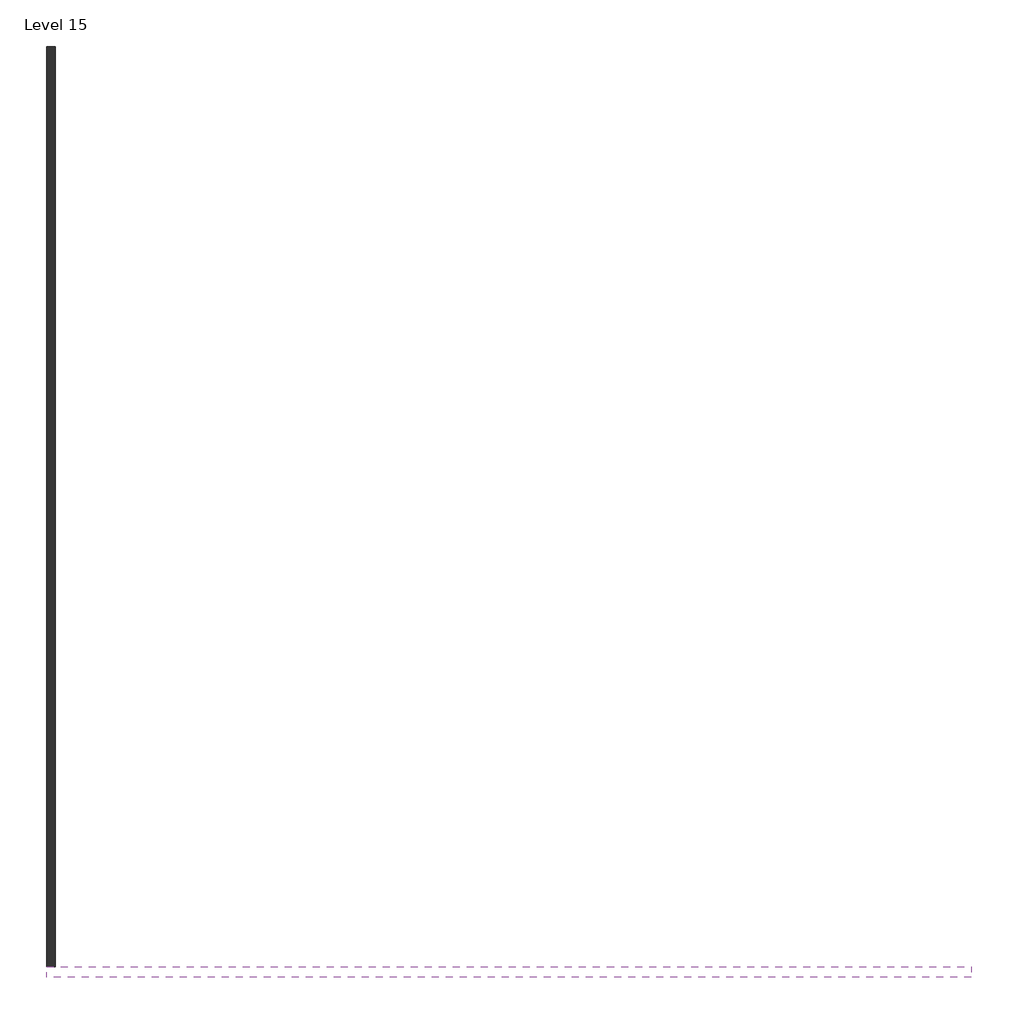
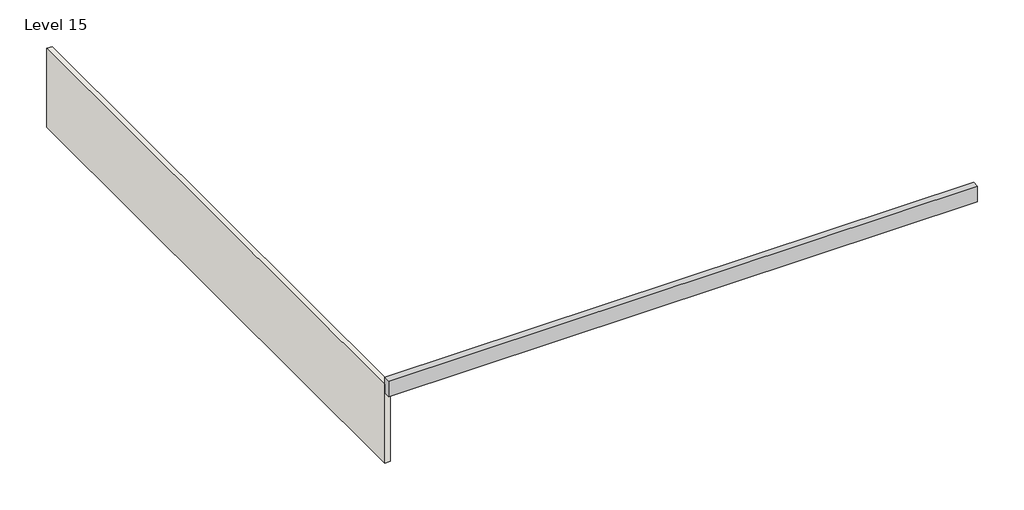
# One storey: 1 proxy, 1 wall.
"""IFC4 building model written with IfcOpenShell, lengths in millimetres."""

from ifc_helpers import new_model, si_unit, origin, place, context, project, spatial, faceted_brep, transform, mapped, element, save
from components import generic_models_10_generic_models_10_516a4994

model = new_model("IFC4")

# Units and contexts
model_context = context("Model", 3, world=origin())
ifc_project = project(units=[si_unit("LENGTHUNIT", "METRE", prefix="MILLI")], contexts=[model_context])

# Site, building, storey
site = spatial("IfcSite", under=ifc_project)
building = spatial("IfcBuilding", under=site)
storey = spatial("IfcBuildingStorey", under=building, Name="Level 15", Elevation=22936.2)

# Proxy
placement = place(None, origin())
generic_models_10_generic_models_10_shape = generic_models_10_generic_models_10_516a4994(model_context)
element("IfcBuildingElementProxy", 1, Name="Generic Models 10 : Generic Models 10", ObjectType="Generic Models 10 : Generic Models 10", at=placement, inside=storey, context=model_context, shape_type="MappedRepresentation", body=[
    mapped(generic_models_10_generic_models_10_shape, transform((0.0, 0.0, 0.0), x_axis=(1.0, 0.0, 0.0), y_axis=(0.0, 1.0, 0.0), z_axis=(0.0, 0.0, 1.0))),
])

# Wall
element("IfcWall", 2, ObjectType="outer wall", at=placement, inside=storey, context=model_context, shape_type="Brep", body=[
    faceted_brep([(-8731.5629849, -3682.5004242, 22936.2), (-8731.5629849, 17551.8995758, 22936.2), (-8731.5629849, 17755.0995758, 22936.2), (-8731.5629849, 17755.0995758, 25984.2), (-8731.5629849, 17551.8995758, 25984.2), (-8731.5629849, -3682.5004242, 25984.2), (-8934.7629849, -3682.5004242, 22936.2), (-8934.7629849, -3682.5004242, 25984.2), (-8934.7629849, 17755.0995758, 25984.2), (-8934.7629849, 17755.0995758, 22936.2), (-8934.7629849, 17551.8995758, 22936.2)], [[[0, 1, 2, 3, 4, 5]], [[6, 7, 8, 9, 10]], [[2, 1, 0, 6, 10, 9]], [[0, 5, 7, 6]], [[5, 4, 3, 8, 7]], [[3, 2, 9, 8]]]),
])

save(model, "model.ifc")

# Revit data of these elements
# Type "outer wall"
#   Assembly Code = "B2010"
#   Layers, outside or top first: 0' - 8" "Copper" (function 1)
# Element 1 (IfcBuildingElementProxy, "Generic Models 10 : Generic Models 10")
#   Phase Created = New Construction
# Element 2 (IfcWall, "outer wall")
#   Top Offset = 0' - 0"
#   Base Offset = 0' - 0"
#   Unconnected Height = 10' - 0"
#   wall height = 10' - 0"
#   Phase Created = New Construction
#   Base Constraint = Level 15
#   Materials on its faces: "Copper"
# Materials
#   "Copper": class "Metal", colour RGB 0 0 0, transparency 0, Description = "Copper, matte finish", Cost = 0
